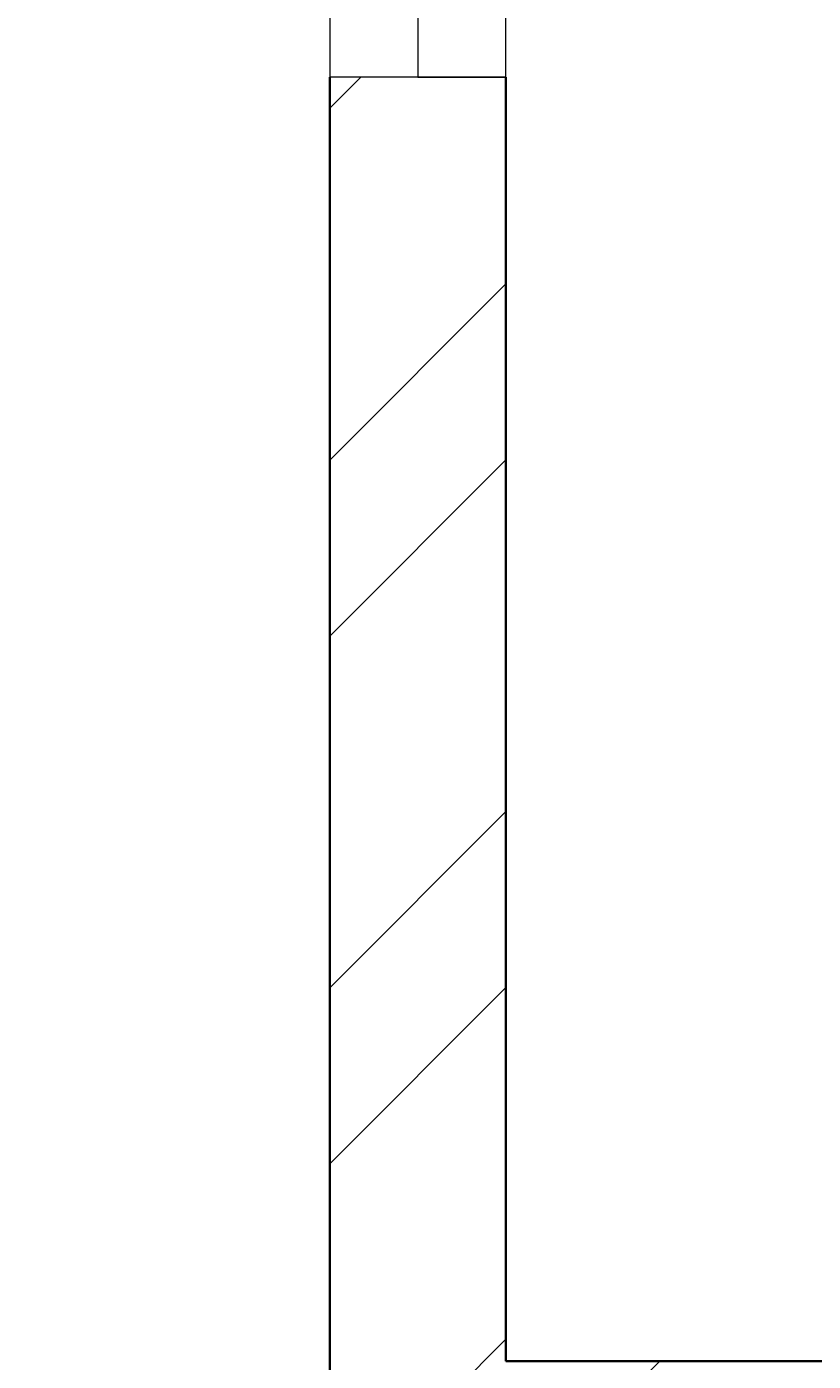
# Model space of a CAD drawing. Units: inches. Extents: x 1885 to 2748, y 783 to 2421.
# Tile 59 of 117: x 2009 to 2029, y 1886 to 1920. Entities that reach past the tile are written whole.
import ezdxf

# ---------------------------------------------------------------- set-up
doc = ezdxf.new("R2010")
doc.units = ezdxf.units.IN
for name, color, linetype, lineweight in [('A-ANNO-DIMS', 2, 'Continuous', 18), ('A-GLAZ', 181, 'Continuous', 18), ('A-WALL', 7, 'Continuous', 35)]:
    doc.layers.add(name, color=color, linetype=linetype, lineweight=lineweight)
doc.layers.add('A-WALL-PATT', color=85, linetype='Continuous', lineweight=13, true_color=0x58ba48)
doc.styles.get("Standard").update_dxf_attribs({"font": 'arial.ttf'})
doc.dimstyles.get("Standard").update_dxf_attribs({"dimtxt": 0.18, "dimasz": 0.18, "dimexe": 0.18, "dimexo": 0.0625, "dimgap": 0.09, "dimtad": 0, "dimtih": 1, "dimtoh": 1, "dimdec": 4, "dimzin": 0, "dimdsep": 46, "dimtxsty": 'Standard', "dimcen": 0.09, "dimadec": 0, "dimazin": 0, "dimtfac": 1, "dimtdec": 4, "dimtofl": 0, "dimtmove": 0, "dimatfit": 3, "dimfxl": 1, "dimtolj": 1, "dimtzin": 0, "dimarcsym": 0})

# ---------------------------------------------------------------- blocks, each defined once
blk = doc.blocks.new('WIN-60-ALT')
for p, q in [((0.004, 59.998), (0.004, -0.002)), ((2.254, 59.998), (2.254, -0.002)), ((4.504, -0.002), (4.504, 59.998)), ((4.504, -0.002), (0.004, -0.002)), ((2.254, -0.002), (4.504, -0.002))]:
    blk.add_line(p, q)
blk = doc.blocks.new('*D48')
at = {"layer": 'A-ANNO-DIMS', "color": 0, "lineweight": -2, "transparency": 16777216}
for p, q in [((1980.711, 2348.006), (1902.844, 2348.006)), ((1903.024, 2347.826), (1903.024, 2114.937)), ((1903.024, 1881.686), (1903.024, 2114.574)), ((2016.711, 1881.506), (1902.844, 1881.506))]:
    blk.add_line(p, q, dxfattribs=at)
at = {"layer": 'A-ANNO-DIMS', "color": 0, "transparency": 16777216}
for points in [[(1902.994, 2347.826), (1903.054, 2347.826), (1903.024, 2348.006)], [(1902.994, 1881.686), (1903.054, 1881.686), (1903.024, 1881.506)]]:
    blk.add_solid(points, dxfattribs=at)
at = {"layer": 'Defpoints', "color": 0, "transparency": 16777216}
for p in [(1903.024, 2348.006), (1980.774, 2348.006), (2016.774, 1881.506)]:
    blk.add_point(p, dxfattribs=at)
at = {"layer": 'A-ANNO-DIMS', "color": 0, "transparency": 16777216, "insert": (1903.024, 2114.756), "char_height": 0.18, "attachment_point": 5}
blk.add_mtext('\\A1;466.5', dxfattribs=at)

msp = doc.modelspace()

# ---------------------------------------------------------------- hatches: boundary and pattern name
at = {"layer": 'A-WALL-PATT'}
h = msp.add_hatch(dxfattribs=at)
h.set_pattern_fill('ANSI32', color=256)
h.paths.add_polyline_path([(2007.772, 2318.006), (1980.774, 2318.006), (1980.774, 2281.215), (1985.274, 2281.215), (1985.274, 2313.506), (2007.772, 2313.506), (2007.772, 2315.756)])
h.paths.add_polyline_path([(2094.324, 2318.006), (2067.772, 2318.006), (2067.772, 2313.506), (2094.324, 2313.506), (2094.324, 2315.756)])
h.paths.add_polyline_path([(2131.367, 2315.756), (2131.367, 2318.006), (2131.189, 2318.006), (2112.609, 2318.006), (2112.609, 2313.506), (2117.274, 2313.506), (2117.274, 2255.201), (2121.774, 2255.201), (2121.774, 2313.506), (2131.367, 2313.506)])
h.paths.add_polyline_path([(2190.512, 2318.006), (2155.367, 2318.006), (2155.367, 2313.506), (2169.774, 2313.506), (2169.774, 2229.506), (2121.774, 2229.506), (2121.774, 2233.451), (2119.524, 2233.451), (2117.274, 2233.451), (2117.274, 2201.101), (2121.774, 2201.101), (2121.774, 2225.006), (2169.774, 2225.006), (2169.774, 2165.006), (2306.274, 2165.006), (2306.274, 2066.006), (2310.774, 2066.006), (2344.274, 2066.006), (2486.274, 2066.006), (2486.274, 1886.006), (2483.02, 1886.006), (2483.02, 1881.506), (2486.274, 1881.506), (2486.274, 1880.678), (2490.774, 1880.678), (2490.774, 2070.506), (2344.274, 2070.506), (2310.774, 2070.506), (2310.774, 2165.006), (2310.774, 2173.636), (2308.524, 2173.636), (2306.274, 2173.636), (2306.274, 2169.506), (2174.274, 2169.506), (2174.274, 2313.506), (2190.512, 2313.506), (2190.512, 2315.756)])
h.paths.add_polyline_path([(1985.274, 2221.215), (1980.774, 2221.215), (1980.774, 2165.006), (1992.774, 2165.006), (1992.774, 2141.927), (1997.274, 2141.927), (1997.274, 2165.006), (2117.274, 2165.006), (2117.274, 2163.126), (2121.774, 2163.126), (2121.774, 2172.734), (2119.524, 2172.734), (2117.274, 2172.734), (2117.274, 2169.506), (1985.274, 2169.506)])
h.paths.add_polyline_path([(1997.274, 2105.927), (1992.774, 2105.927), (1992.774, 2070.506), (2016.774, 2070.506), (2016.774, 2059.123), (2019.024, 2059.123), (2021.274, 2059.123), (2021.274, 2070.506), (2117.274, 2070.506), (2117.274, 2022.506), (2114.423, 2022.506), (2114.423, 2018.006), (2123.627, 2018.006), (2123.627, 2020.256), (2123.627, 2022.506), (2121.774, 2022.506), (2121.774, 2142.587), (2119.524, 2142.587), (2117.274, 2142.587), (2117.274, 2075.006), (1997.274, 2075.006)])
h.paths.add_polyline_path([(2092.029, 2020.256), (2092.029, 2022.506), (2021.274, 2022.506), (2021.274, 2035.123), (2016.774, 2035.123), (2016.774, 2018.006), (2016.774, 1978.784), (2021.274, 1978.784), (2021.274, 2018.006), (2092.029, 2018.006)])
h.paths.add_polyline_path([(2260.938, 2022.506), (2153.105, 2022.506), (2153.105, 2020.256), (2153.105, 2018.006), (2155.274, 2018.006), (2155.274, 1886.006), (2107.629, 1886.006), (2107.629, 1881.506), (2182.911, 1881.506), (2182.911, 1883.756), (2182.911, 1886.006), (2159.774, 1886.006), (2159.774, 2018.006), (2260.938, 2018.006), (2260.938, 2020.256)])
h.paths.add_polyline_path([(2047.629, 1883.756), (2047.629, 1886.006), (2021.274, 1886.006), (2021.274, 1918.784), (2019.024, 1918.784), (2016.774, 1918.784), (2016.774, 1881.506), (2047.629, 1881.506)])
h.paths.add_polyline_path([(2306.361, 1883.756), (2306.361, 1886.006), (2296.274, 1886.006), (2296.274, 1982.006), (2316.535, 1982.006), (2316.535, 1984.256), (2316.535, 1986.506), (2296.274, 1986.506), (2296.274, 2022.506), (2289.276, 2022.506), (2289.276, 2018.006), (2291.774, 2018.006), (2291.774, 1886.006), (2242.911, 1886.006), (2242.911, 1881.506), (2306.361, 1881.506)], flags=17)
h.paths.add_polyline_path([(1985.274, 1843.006), (2021.6, 1843.006), (2021.534, 1845.441), (2021.477, 1847.506), (1980.774, 1847.506), (1980.774, 1809.446), (1985.274, 1809.446)])
h.paths.add_polyline_path([(2131.482, 1845.256), (2131.482, 1847.506), (2081.534, 1847.506), (2081.534, 1843.006), (2117.274, 1843.006), (2117.274, 1784.147), (2119.524, 1784.147), (2121.774, 1784.147), (2121.774, 1843.006), (2131.482, 1843.006)])
h.paths.add_polyline_path([(2203.886, 1847.506), (2155.482, 1847.506), (2155.482, 1843.006), (2169.774, 1843.006), (2169.774, 1759.006), (2121.774, 1759.006), (2121.774, 1761.457), (2117.274, 1761.457), (2117.274, 1730.429), (2121.774, 1730.429), (2121.774, 1754.506), (2177.421, 1754.506), (2177.421, 1756.756), (2177.421, 1759.006), (2174.274, 1759.006), (2174.274, 1843.006), (2203.886, 1843.006)])
h.paths.add_polyline_path([(2335.554, 1845.256), (2335.554, 1847.506), (2239.886, 1847.506), (2239.886, 1843.006), (2306.274, 1843.006), (2306.274, 1759.006), (2199.486, 1759.006), (2199.486, 1754.506), (2310.774, 1754.506), (2310.774, 1843.006), (2335.554, 1843.006)])
h.paths.add_polyline_path([(2348.774, 2022.506), (2344.274, 2022.506), (2344.274, 1986.506), (2341.681, 1986.506), (2341.681, 1982.006), (2344.274, 1982.006), (2344.274, 1886.006), (2330.361, 1886.006), (2330.361, 1881.506), (2361.627, 1881.506), (2361.627, 1883.756), (2361.627, 1886.006), (2348.774, 1886.006)], flags=17)
h.paths.add_polyline_path([(2283.251, 2315.756), (2283.251, 2318.006), (2238.512, 2318.006), (2238.512, 2313.506), (2283.251, 2313.506)], flags=17)
h.paths.add_polyline_path([(2363.274, 2348.006), (2388.677, 2348.006), (2388.677, 2350.256), (2388.677, 2352.506), (2358.774, 2352.506), (2358.774, 2348.006), (2358.774, 2318.006), (2344.481, 2318.006), (2344.481, 2313.506), (2358.774, 2313.506), (2358.774, 2229.506), (2310.774, 2229.506), (2310.774, 2231.952), (2306.274, 2231.952), (2306.274, 2205.611), (2310.774, 2205.611), (2310.774, 2225.006), (2358.774, 2225.006), (2358.774, 2211.506), (2452.329, 2211.506), (2452.329, 2213.756), (2452.329, 2216.006), (2363.274, 2216.006), (2363.274, 2318.006)])
h.paths.add_polyline_path([(2310.774, 2313.506), (2320.481, 2313.506), (2320.481, 2315.756), (2320.481, 2318.006), (2302.728, 2318.006), (2302.728, 2313.506), (2306.274, 2313.506), (2306.274, 2251.076), (2310.774, 2251.076)], flags=17)
h.paths.add_polyline_path([(2490.774, 2352.506), (2486.274, 2352.506), (2448.677, 2352.506), (2448.677, 2348.006), (2486.274, 2348.006), (2486.274, 2318.006), (2486.274, 2216.006), (2481.78, 2216.006), (2481.78, 2211.506), (2486.274, 2211.506), (2486.274, 2165.006), (2493.289, 2165.006), (2493.289, 2167.256), (2493.289, 2169.506), (2490.774, 2169.506), (2490.774, 2313.506), (2494.429, 2313.506), (2494.429, 2318.006), (2490.774, 2318.006)])
h.paths.add_polyline_path([(2534.653, 2318.006), (2515.691, 2318.006), (2515.691, 2313.506), (2534.653, 2313.506), (2534.653, 2315.756)])
h.paths.add_polyline_path([(2618.274, 2318.006), (2594.653, 2318.006), (2594.653, 2313.506), (2613.774, 2313.506), (2613.774, 2281.706), (2618.274, 2281.706)])
h.paths.add_polyline_path([(2618.274, 2221.706), (2613.774, 2221.706), (2613.774, 2169.506), (2554.019, 2169.506), (2554.019, 2165.006), (2613.774, 2165.006), (2613.774, 2152.878), (2618.274, 2152.878)])
h.paths.add_polyline_path([(2618.274, 2128.878), (2616.024, 2128.878), (2613.774, 2128.878), (2613.774, 2117.006), (2529.774, 2117.006), (2529.774, 2165.006), (2532.848, 2165.006), (2532.848, 2169.506), (2522.867, 2169.506), (2522.867, 2165.006), (2525.274, 2165.006), (2525.274, 2117.006), (2525.274, 2112.506), (2525.274, 2108.576), (2529.774, 2108.576), (2529.774, 2112.506), (2613.774, 2112.506), (2613.774, 2080.19), (2618.274, 2080.19)])
h.paths.add_polyline_path([(2618.274, 2044.19), (2616.024, 2044.19), (2613.774, 2044.19), (2613.774, 2015.506), (2529.774, 2015.506), (2529.774, 2088.582), (2527.524, 2088.582), (2525.274, 2088.582), (2525.274, 2011.006), (2613.774, 2011.006), (2613.774, 1956.755), (2618.274, 1956.755)])
h.paths.add_polyline_path([(2618.274, 1881.506), (2618.274, 1896.755), (2613.774, 1896.755), (2613.774, 1881.506), (2613.774, 1847.506), (2592.715, 1847.506), (2592.715, 1843.006), (2613.774, 1843.006), (2613.774, 1765.006), (2613.774, 1760.506), (2609.621, 1760.506), (2609.621, 1756.006), (2613.774, 1756.006), (2613.774, 1660.006), (2608.544, 1660.006), (2608.544, 1655.506), (2613.774, 1655.506), (2613.774, 1508.158), (2618.274, 1508.158)])
h.paths.add_polyline_path([(2565.774, 1843.006), (2568.997, 1843.006), (2568.997, 1847.506), (2490.774, 1847.506), (2490.774, 1849.7), (2488.524, 1849.7), (2486.274, 1849.7), (2486.274, 1847.506), (2477.274, 1847.506), (2477.274, 1838.506), (2477.274, 1821.493), (2486.274, 1821.493), (2486.274, 1838.506), (2561.274, 1838.506), (2561.274, 1765.006), (2486.274, 1765.006), (2486.274, 1786.157), (2477.274, 1786.157), (2477.274, 1765.006), (2477.274, 1756.006), (2486.274, 1756.006), (2565.774, 1756.006), (2585.621, 1756.006), (2585.621, 1758.256), (2585.621, 1760.506), (2565.774, 1760.506), (2565.774, 1765.006)])
h.paths.add_polyline_path([(2486.274, 1651.006), (2561.274, 1651.006), (2561.274, 1567.006), (2486.274, 1567.006), (2486.274, 1591.321), (2477.274, 1591.321), (2477.274, 1567.006), (2477.274, 1558.006), (2477.274, 1555.439), (2481.774, 1555.439), (2481.774, 1558.006), (2568.653, 1558.006), (2568.653, 1560.256), (2568.653, 1562.506), (2565.774, 1562.506), (2565.774, 1655.506), (2584.544, 1655.506), (2584.544, 1657.756), (2584.544, 1660.006), (2565.774, 1660.006), (2486.274, 1660.006), (2477.274, 1660.006), (2477.274, 1651.006), (2477.274, 1632.989), (2486.274, 1632.989)])
h.paths.add_polyline_path([(2449.967, 1883.756), (2449.967, 1886.006), (2421.627, 1886.006), (2421.627, 1881.506), (2449.967, 1881.506)], flags=17)
h.paths.add_polyline_path([(2447.274, 1847.506), (2395.554, 1847.506), (2395.554, 1843.006), (2442.774, 1843.006), (2442.774, 1809.27), (2447.274, 1809.27)])
h.paths.add_polyline_path([(1985.274, 1749.446), (1980.774, 1749.446), (1980.774, 1694.504), (1985.274, 1694.504), (1985.274, 1694.506), (1986.897, 1694.506), (1986.897, 1697.78), (1986.897, 1699.006), (1985.274, 1699.006)])
h.paths.add_polyline_path([(2152.774, 1699.006), (2121.774, 1699.006), (2121.774, 1703.668), (2119.524, 1703.668), (2117.274, 1703.668), (2117.274, 1699.006), (2009.219, 1699.006), (2009.219, 1694.506), (2148.274, 1694.506), (2148.274, 1692.631), (2152.774, 1692.631)])
h.paths.add_polyline_path([(2016.274, 1694.506), (2011.774, 1694.506), (2011.774, 1558.006), (2040.806, 1558.006), (2040.806, 1560.256), (2040.806, 1562.506), (2016.274, 1562.506)])
h.paths.add_polyline_path([(2152.774, 1663.017), (2150.524, 1663.017), (2148.274, 1663.017), (2148.274, 1562.506), (2100.806, 1562.506), (2100.806, 1558.006), (2165.119, 1558.006), (2165.119, 1560.256), (2165.119, 1562.506), (2152.774, 1562.506), (2152.774, 1610.506), (2224.774, 1610.506), (2224.774, 1607.99), (2229.274, 1607.99), (2229.274, 1615.006), (2152.774, 1615.006)])
h.paths.add_polyline_path([(2238.613, 1560.256), (2238.613, 1562.506), (2229.274, 1562.506), (2229.274, 1588.756), (2227.024, 1588.763), (2224.774, 1588.771), (2224.774, 1562.506), (2189.119, 1562.506), (2189.119, 1558.006), (2238.613, 1558.006)])
h.paths.add_polyline_path([(2336.024, 1560.256), (2336.024, 1562.506), (2310.774, 1562.506), (2310.774, 1656.347), (2308.524, 1656.347), (2306.274, 1656.347), (2306.274, 1562.506), (2286.613, 1562.506), (2286.613, 1558.006), (2336.024, 1558.006)])
h.paths.add_polyline_path([(2447.274, 1690.968), (2445.024, 1690.968), (2442.774, 1690.968), (2442.774, 1687.006), (2306.274, 1687.006), (2306.274, 1680.75), (2310.774, 1680.75), (2310.774, 1682.506), (2442.774, 1682.506), (2442.774, 1562.506), (2396.024, 1562.506), (2396.024, 1558.006), (2447.274, 1558.006)])
h.paths.add_polyline_path([(2447.274, 1749.27), (2445.024, 1749.27), (2442.774, 1749.27), (2442.774, 1717.232), (2447.274, 1717.232)])
h.paths.add_polyline_path([(2044.674, 1521.756), (2044.674, 1524.006), (2007.274, 1524.006), (2007.274, 1503.49), (2009.524, 1503.49), (2011.774, 1503.49), (2011.774, 1519.506), (2044.674, 1519.506)])
h.paths.add_polyline_path([(2177.969, 1521.756), (2177.969, 1524.006), (2104.674, 1524.006), (2104.674, 1519.506), (2145.774, 1519.506), (2145.774, 1387.506), (2143.37, 1387.506), (2143.37, 1383.006), (2251.585, 1383.006), (2251.585, 1385.256), (2251.585, 1387.506), (2150.274, 1387.506), (2150.274, 1519.506), (2177.969, 1519.506)])
h.paths.add_polyline_path([(2298.704, 1524.006), (2237.969, 1524.006), (2237.969, 1519.506), (2282.274, 1519.506), (2282.274, 1387.506), (2279.683, 1387.506), (2279.683, 1383.006), (2286.774, 1383.006), (2286.774, 1419.006), (2312.451, 1419.006), (2312.451, 1421.256), (2312.451, 1423.506), (2286.774, 1423.506), (2286.774, 1519.506), (2298.704, 1519.506), (2298.704, 1521.722)], flags=17)
h.paths.add_polyline_path([(2361.897, 1521.756), (2361.897, 1524.006), (2322.704, 1524.006), (2322.704, 1519.506), (2334.774, 1519.506), (2334.774, 1423.506), (2331.93, 1423.506), (2331.93, 1419.006), (2334.774, 1419.006), (2334.774, 1387.506), (2334.774, 1383.228), (2339.274, 1383.228), (2339.274, 1387.506), (2339.274, 1519.506), (2361.897, 1519.506)], flags=17)
h.paths.add_polyline_path([(2447.274, 1521.756), (2447.274, 1524.006), (2421.897, 1524.006), (2421.897, 1519.506), (2447.274, 1519.506)], flags=17)
h.paths.add_polyline_path([(2481.774, 1529.6), (2479.524, 1529.6), (2477.274, 1529.6), (2477.274, 1524.006), (2474.489, 1524.006), (2474.489, 1519.506), (2477.274, 1519.506), (2477.274, 1334.506), (2296.774, 1334.506), (2296.774, 1240.506), (2160.274, 1240.506), (2160.274, 1180.506), (2112.274, 1180.506), (2112.274, 1207.692), (2110.024, 1207.692), (2107.774, 1207.692), (2107.774, 1171.609), (2112.274, 1171.609), (2112.274, 1176.006), (2160.274, 1176.006), (2160.274, 1092.006), (2144.221, 1092.006), (2144.221, 1087.506), (2189.497, 1087.506), (2189.497, 1089.756), (2189.497, 1092.006), (2164.774, 1092.006), (2164.774, 1236.006), (2296.774, 1236.006), (2296.774, 1231.912), (2301.274, 1231.912), (2301.274, 1330.006), (2481.774, 1330.006), (2481.774, 1387.506)])
h.paths.add_polyline_path([(2618.274, 1448.158), (2613.774, 1448.158), (2613.774, 1382.506), (2529.774, 1382.506), (2525.274, 1382.506), (2525.274, 1307.062), (2529.774, 1307.062), (2529.774, 1378.006), (2613.774, 1378.006), (2613.774, 1354.988), (2618.274, 1354.988)])
h.paths.add_polyline_path([(2618.274, 1318.988), (2613.774, 1318.988), (2613.774, 1281.006), (2529.774, 1281.006), (2529.774, 1283.786), (2527.524, 1283.786), (2525.274, 1283.786), (2525.274, 1228.506), (2516.794, 1228.506), (2516.794, 1224.006), (2533.484, 1224.006), (2533.484, 1226.256), (2533.484, 1228.506), (2529.774, 1228.506), (2529.774, 1276.506), (2613.774, 1276.506), (2613.774, 1266.02), (2618.274, 1266.02)])
h.paths.add_polyline_path([(2618.274, 1134.964), (2613.774, 1134.964), (2613.774, 1092.006), (2594.545, 1092.006), (2594.545, 1087.506), (2618.274, 1087.506)])
h.paths.add_polyline_path([(2534.545, 1092.006), (2509.765, 1092.006), (2509.765, 1087.506), (2534.545, 1087.506), (2534.545, 1089.756)])
h.paths.add_polyline_path([(2481.274, 1224.006), (2484.117, 1224.006), (2484.117, 1226.256), (2484.117, 1228.506), (2476.774, 1228.506), (2476.774, 1198.506), (2471.61, 1198.506), (2471.61, 1194.006), (2476.774, 1194.006), (2476.774, 1062.006), (2436.894, 1062.006), (2436.894, 1057.506), (2476.774, 1057.506), (2481.274, 1057.506), (2481.274, 1062.006), (2481.274, 1087.506), (2485.354, 1087.506), (2485.354, 1089.756), (2485.354, 1092.006), (2481.274, 1092.006), (2481.274, 1117.506)])
h.paths.add_polyline_path([(2439.898, 1198.506), (2349.274, 1198.506), (2349.274, 1194.006), (2349.274, 1180.506), (2301.274, 1180.506), (2301.274, 1201.896), (2299.024, 1201.896), (2296.774, 1201.896), (2296.774, 1172.335), (2299.024, 1172.335), (2301.274, 1172.335), (2301.274, 1176.006), (2349.274, 1176.006), (2349.274, 1092.006), (2334.452, 1092.006), (2334.452, 1087.506), (2349.274, 1087.506), (2349.274, 1057.506), (2353.774, 1057.506), (2376.894, 1057.506), (2376.894, 1059.756), (2376.894, 1062.006), (2353.774, 1062.006), (2353.774, 1087.506), (2353.774, 1180.506), (2353.774, 1194.006), (2439.898, 1194.006), (2439.898, 1196.256)])
h.paths.add_polyline_path([(2270.596, 1089.756), (2270.596, 1092.006), (2249.497, 1092.006), (2249.497, 1087.506), (2270.596, 1087.506)], flags=17)
h.paths.add_polyline_path([(2310.452, 1092.006), (2301.274, 1092.006), (2301.274, 1153.292), (2296.774, 1153.292), (2296.774, 1092.006), (2293.786, 1092.006), (2293.786, 1087.506), (2310.452, 1087.506), (2310.452, 1089.756)], flags=17)
h.paths.add_polyline_path([(2112.274, 1150.328), (2110.024, 1150.328), (2107.774, 1150.328), (2107.774, 1092.006), (2104.465, 1092.006), (2104.465, 1087.506), (2120.221, 1087.506), (2120.221, 1089.756), (2120.221, 1092.006), (2112.274, 1092.006)])
h.paths.add_polyline_path([(2082.172, 1092.006), (2058.144, 1092.006), (2058.144, 1087.506), (2082.172, 1087.506), (2082.172, 1089.756)])
h.paths.add_polyline_path([(1975.774, 1145.638), (1971.274, 1145.638), (1971.274, 1087.506), (1980.774, 1087.506), (1998.144, 1087.506), (1998.144, 1089.756), (1998.144, 1092.006), (1985.274, 1092.006), (1975.774, 1092.006)])
h.paths.add_polyline_path([(2112.274, 1244.385), (2110.024, 1244.385), (2107.774, 1244.385), (2107.774, 1240.506), (1992.274, 1240.506), (1992.274, 1271.008), (1987.774, 1271.008), (1987.774, 1240.506), (1980.774, 1240.506), (1975.774, 1240.506), (1971.274, 1240.506), (1971.274, 1205.638), (1975.774, 1205.638), (1975.774, 1236.006), (2107.774, 1236.006), (2107.774, 1233.444), (2112.274, 1233.444), (2112.274, 1236.006)])
h.paths.add_polyline_path([(2112.274, 1383.006), (2114.783, 1383.006), (2114.783, 1385.256), (2114.783, 1387.506), (2102.476, 1387.506), (2102.476, 1383.006), (2107.774, 1383.006), (2107.774, 1335.006), (2011.774, 1335.006), (2011.774, 1349.939), (2007.274, 1349.939), (2007.274, 1335.006), (1987.774, 1335.006), (1987.774, 1330.506), (1987.774, 1307.008), (1992.274, 1307.008), (1992.274, 1330.506), (2007.274, 1330.506), (2107.774, 1330.506), (2107.774, 1264.711), (2112.274, 1264.711)])
h.paths.add_polyline_path([(2077.857, 1387.506), (2011.774, 1387.506), (2011.774, 1390.036), (2009.524, 1390.036), (2007.274, 1390.036), (2007.274, 1373.939), (2011.774, 1373.939), (2011.774, 1383.006), (2077.857, 1383.006)])
h.paths.add_polyline_path([(2011.774, 1443.49), (2007.274, 1443.49), (2007.274, 1410.248), (2011.774, 1410.248)])

# ---------------------------------------------------------------- linework, layer by layer
at = {"layer": 'A-WALL'}
for p, q in [((2016.774, 1918.784), (2016.774, 1881.506)), ((2021.274, 1886.006), (2021.274, 1918.784)), ((2021.274, 1886.006), (2047.629, 1886.006))]:
    msp.add_line(p, q, dxfattribs=at)

# ---------------------------------------------------------------- block references
at = {"layer": 'A-GLAZ'}
msp.add_blockref('WIN-60-ALT', (2016.77, 1918.787), dxfattribs=at)

# ---------------------------------------------------------------- dimensions: what is measured, and where the dimension line sits
at = {"layer": 'A-ANNO-DIMS'}
dim = msp.add_linear_dim(base=(1903.024, 2348.006), p1=(2016.774, 1881.506), p2=(1980.774, 2348.006), angle=90, dimstyle='Standard', override={"dimdec": 1, "dimlfac": 1, "dimrnd": 0, "dimzin": 0, "dimdsep": 46, "dimlunit": 2}, dxfattribs=at)
dim.commit()
dim.dimension.update_dxf_attribs({"geometry": '*D48', "text_midpoint": (1903.024, 2114.756)})

doc.saveas('drawing.dxf')
